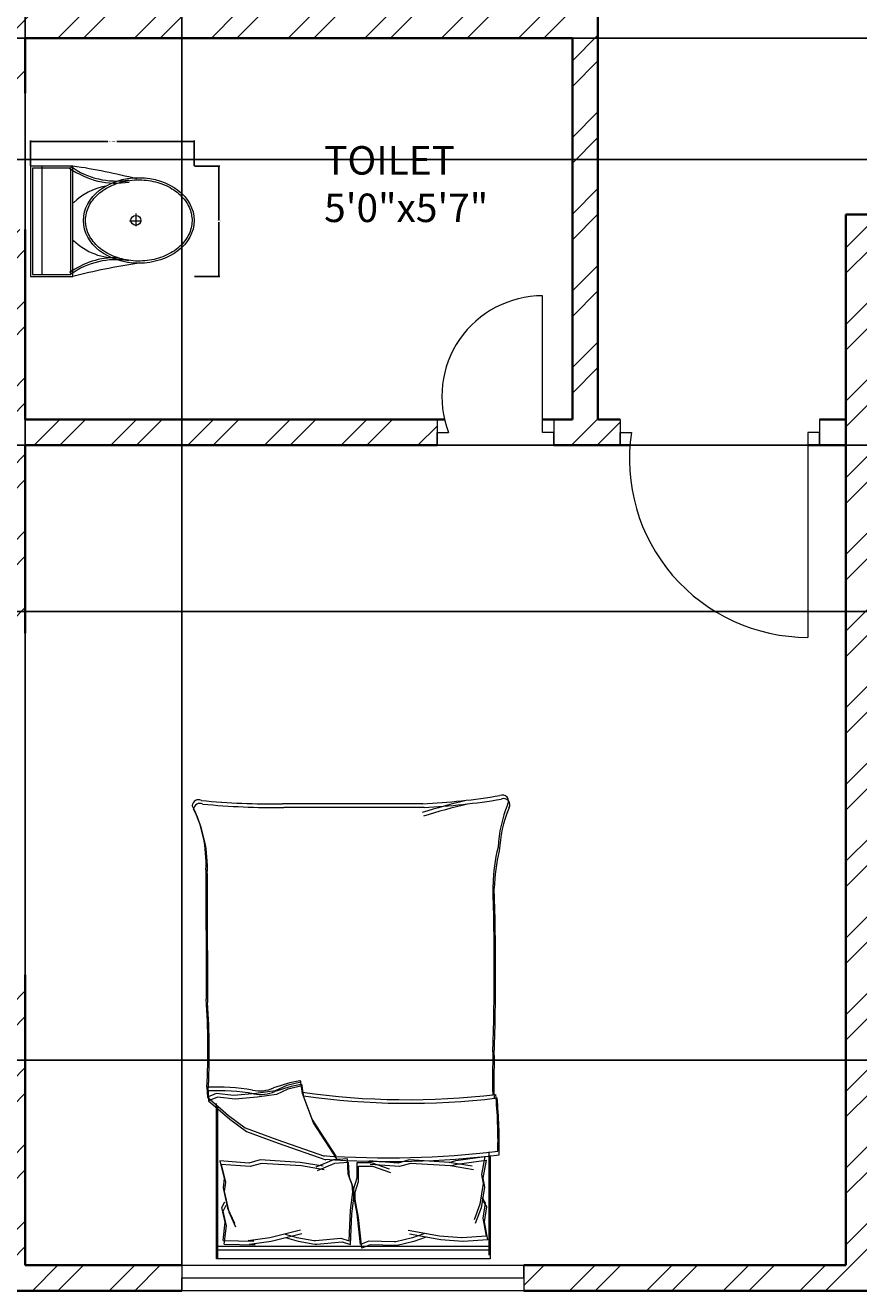
# Model space of a CAD drawing. Units: inches. Extents: x 1965 to 2673, y 1802 to 2669.
# Tile 3 of 16: x 2052 to 2198, y 1932 to 2154. Entities that reach past the tile are written whole.
import ezdxf

# ---------------------------------------------------------------- set-up
doc = ezdxf.new("R2010")
doc.units = ezdxf.units.IN
for name, color, linetype, lineweight in [('A-ANNO-DIMS', 2, 'Continuous', 18), ('A-AREA-IDEN', 7, 'Continuous', 18), ('A-DOOR', 11, 'Continuous', 18), ('A-FLOR-FIXT', 9, 'Continuous', 18), ('A-FURN', 8, 'Continuous', 13), ('A-GLAZ', 181, 'Continuous', 18), ('A-WALL', 7, 'Continuous', 35), ('A-WALL-PATT', 252, 'Continuous', 13)]:
    doc.layers.add(name, color=color, linetype=linetype, lineweight=lineweight)
doc.styles.get("Standard").update_dxf_attribs({"font": 'arial.ttf'})
doc.dimstyles.get("Standard").update_dxf_attribs({"dimtxt": 0.18, "dimasz": 0.18, "dimexe": 0.18, "dimexo": 0.0625, "dimgap": 0.09, "dimtad": 0, "dimtih": 1, "dimtoh": 1, "dimdec": 4, "dimzin": 0, "dimdsep": 46, "dimtxsty": 'Standard', "dimcen": 0.09, "dimadec": 0, "dimazin": 0, "dimtfac": 1, "dimtdec": 4, "dimtofl": 0, "dimtmove": 0, "dimatfit": 3, "dimfxl": 1, "dimtolj": 1, "dimtzin": 0, "dimarcsym": 0})

# ---------------------------------------------------------------- blocks, each defined once
blk = doc.blocks.new('A$C31115884')
for p, q in [((283.1, 497.7), (223.4, 497.7)), ((257.5, 466.4), (257.5, 523.2)), ((0, 200), (0, 0)), ((520, 200), (0, 200)), ((10, 190), (10, 10)), ((510, 190), (10, 190)), ((510, 10), (510, 190)), ((520, 0), (520, 200)), ((510, 54.5), (0, 54.5)), ((10, 10), (510, 10)), ((0, 0), (520, 0))]:
    blk.add_line(p, q)
blk.add_circle((255.6, 496.4), 23.6)
for centre, radius, start, end in [((2777.7, -204.6), 2807, 165.4549, 171.71327), ((3237, 905), 2807, 188.28673, 194.5451), ((-294.5, 403.3), 364.7, 324.20913, 9.34987), ((-294.5, 403.3), 374.7, 324.20913, 9.34987), ((139.5, 406.2), 293.5, 315.84364, 2.65635), ((805.8, 403.3), 364.7, 170.65013, 215.79087), ((805.8, 403.3), 374.7, 179.20365, 215.79087), ((383.6, 406.2), 293.5, 190.27735, 224.15636)]:
    blk.add_arc(centre, radius, start, end)
blk.add_ellipse((256.2, 509.9), major_axis=(0, -260.7), ratio=0.772727)
blk.add_open_spline([(256.2, 259.2), (263.1, 259.2), (270, 259.7), (287.8, 262.3), (298.7, 265.1), (319.9, 273.1), (330.2, 278.4), (350.1, 291.1), (359.7, 298.7), (377.7, 315.9), (386.2, 325.5), (401.7, 346.6), (408.8, 358.1), (421.3, 382.5), (426.8, 395.5), (435.9, 422.4), (439.5, 436.4), (444.8, 465.1), (446.5, 479.7), (447.9, 509.2), (447.6, 524), (445, 553.3), (442.7, 567.8), (436.3, 596), (432.1, 609.7), (421.9, 636), (416, 648.6), (402.5, 672.1), (395, 683), (378.6, 703), (369.8, 712.1), (351.1, 728), (341.3, 734.8), (320.9, 746.2), (310.4, 750.7), (288.9, 757.3), (278, 759.4), (256, 761), (245, 760.6), (223.1, 757.2), (212.3, 754.3), (191.1, 746.1), (180.8, 740.7), (160.9, 727.8), (151.4, 720.1), (133.5, 702.7), (125.1, 693), (109.6, 671.7), (102.6, 660.2), (90.2, 635.7), (84.9, 622.7), (76, 595.6), (72.4, 581.6), (67.2, 552.9), (65.6, 538.2), (64.4, 508.8), (64.8, 494), (67.5, 464.7), (69.9, 450.2), (76.6, 422), (80.8, 408.3), (91.1, 382.2), (97.2, 369.7), (110.8, 346.3), (118.4, 335.4), (134.8, 315.6), (143.7, 306.7), (162.4, 290.9), (172.3, 284.2), (192.8, 273), (203.3, 268.6), (224.8, 262.2), (235.8, 260.2), (249.9, 259.3), (253, 259.2), (256.2, 259.2)], degree=3, knots=[0, 0, 0, 0, 0.110105, 0.110105, 0.285049, 0.285049, 0.459994, 0.459994, 0.634938, 0.634938, 0.809882, 0.809882, 0.984827, 0.984827, 1.159771, 1.159771, 1.334715, 1.334715, 1.50966, 1.50966, 1.684604, 1.684604, 1.859549, 1.859549, 2.034493, 2.034493, 2.209437, 2.209437, 2.384382, 2.384382, 2.559326, 2.559326, 2.73427, 2.73427, 2.909215, 2.909215, 3.084159, 3.084159, 3.259103, 3.259103, 3.434048, 3.434048, 3.608992, 3.608992, 3.783936, 3.783936, 3.958881, 3.958881, 4.133825, 4.133825, 4.30877, 4.30877, 4.483714, 4.483714, 4.658658, 4.658658, 4.833603, 4.833603, 5.008547, 5.008547, 5.183491, 5.183491, 5.358436, 5.358436, 5.53338, 5.53338, 5.708324, 5.708324, 5.883269, 5.883269, 6.058213, 6.058213, 6.233158, 6.233158, 6.283185, 6.283185, 6.283185, 6.283185])
blk = doc.blocks.new('BED-DOUBLE')
for p, q in [((3.47, 63.33), (3.47, 81.44)), ((3.47, 63.33), (3.47, 81.44)), ((3.47, 81.44), (51.49, 81.44)), ((3.7, 62.69), (3.7, 80.8)), ((3.7, 62.69), (3.7, 80.8)), ((51.26, 81.44), (51.26, 54.83)), ((51.26, 81.44), (51.26, 54.83)), ((51.49, 81.44), (51.49, 80.8)), ((51.49, 80.8), (51.49, 54.19)), ((51.49, 80.8), (51.49, 54.19)), ((3.47, 79.91), (51.26, 79.91)), ((3.47, 79.91), (51.26, 79.91)), ((3.7, 79.27), (51.49, 79.27)), ((3.7, 79.27), (51.49, 79.27)), ((3.89, 78.1), (8.17, 78.43)), ((3.89, 78.1), (8.17, 78.43)), ((3.89, 78.12), (4.47, 74.94)), ((3.89, 78.12), (4.47, 74.94)), ((4.12, 77.46), (8.4, 77.79)), ((4.12, 77.46), (8.4, 77.79)), ((8.17, 78.43), (8.28, 78.41)), ((8.17, 78.43), (8.28, 78.41)), ((8.28, 78.41), (12.1, 78.12)), ((8.28, 78.41), (12.1, 78.12)), ((8.4, 77.79), (8.51, 77.77)), ((8.4, 77.79), (8.51, 77.77)), ((12.1, 78.12), (17.6, 77.11)), ((12.1, 78.12), (17.6, 77.11)), ((14.85, 77.69), (16.87, 78.41)), ((14.85, 77.69), (16.87, 78.41)), ((16.87, 78.41), (19.76, 79.14)), ((16.87, 78.41), (19.76, 79.14)), ((17.1, 77.77), (19.99, 78.5)), ((17.1, 77.77), (19.99, 78.5)), ((19.76, 79.14), (20.09, 79.14)), ((19.76, 79.14), (20.09, 79.14)), ((19.99, 78.5), (20.31, 78.5)), ((19.99, 78.5), (20.31, 78.5)), ((20.09, 79.14), (24.53, 78.99)), ((20.09, 79.14), (24.53, 78.99)), ((20.31, 78.5), (24.76, 78.35)), ((20.31, 78.5), (24.76, 78.35)), ((24.53, 78.99), (25.98, 79.57)), ((24.53, 78.99), (25.98, 79.57)), ((24.76, 78.35), (26.21, 78.93)), ((24.76, 78.35), (26.21, 78.93)), ((25.98, 79.57), (26.56, 74.22)), ((25.98, 79.57), (26.56, 74.22)), ((26.21, 78.93), (26.78, 73.58)), ((26.21, 78.93), (26.78, 73.58)), ((27.97, 78.95), (27.73, 73.57)), ((27.97, 78.95), (27.73, 73.57)), ((28.2, 78.31), (27.96, 72.93)), ((28.2, 78.31), (27.96, 72.93)), ((29.45, 78.46), (27.97, 78.95)), ((29.45, 78.46), (27.97, 78.95)), ((29.68, 77.82), (28.2, 78.31)), ((29.68, 77.82), (28.2, 78.31)), ((33.88, 78.88), (29.45, 78.46)), ((33.88, 78.88), (29.45, 78.46)), ((34.11, 78.24), (29.68, 77.82)), ((34.11, 78.24), (29.68, 77.82)), ((34.2, 78.9), (33.88, 78.88)), ((34.2, 78.9), (33.88, 78.88)), ((34.43, 78.26), (34.11, 78.24)), ((34.43, 78.26), (34.11, 78.24)), ((37.13, 78.36), (34.2, 78.9)), ((37.13, 78.36), (34.2, 78.9)), ((37.36, 77.72), (34.43, 78.26)), ((37.36, 77.72), (34.43, 78.26)), ((41.91, 78.37), (36.49, 77.02)), ((41.91, 78.37), (36.49, 77.02)), ((39.2, 77.77), (37.13, 78.36)), ((39.19, 77.77), (37.13, 78.36)), ((45.71, 78.9), (41.91, 78.37)), ((45.71, 78.9), (41.91, 78.37)), ((45.94, 78.26), (42.14, 77.73)), ((45.94, 78.26), (42.14, 77.73)), ((50.11, 78.88), (44.7, 78.98)), ((44.7, 78.98), (45.71, 78.9)), ((50.11, 78.88), (44.7, 78.98)), ((44.7, 78.98), (45.71, 78.9)), ((50.34, 78.24), (44.93, 78.34)), ((44.93, 78.34), (45.94, 78.26)), ((50.34, 78.24), (44.93, 78.34)), ((44.93, 78.34), (45.94, 78.26)), ((50.11, 78.88), (49.73, 75.67)), ((50.11, 78.88), (49.73, 75.67)), ((50.34, 78.24), (49.96, 75.03)), ((50.34, 78.24), (49.96, 75.03)), ((4.12, 77.49), (4.7, 74.3)), ((4.12, 77.49), (4.7, 74.3)), ((8.51, 77.77), (12.33, 77.49)), ((8.51, 77.77), (12.33, 77.49)), ((12.33, 77.49), (17.82, 76.47)), ((12.33, 77.49), (17.82, 76.47)), ((15.08, 77.05), (17.1, 77.77)), ((15.08, 77.05), (17.1, 77.77)), ((42.14, 77.73), (36.72, 76.38)), ((42.14, 77.73), (36.72, 76.38)), ((39.42, 77.13), (37.36, 77.72)), ((39.42, 77.13), (37.36, 77.72)), ((49.3, 73.18), (48.12, 75.86)), ((49.3, 73.18), (48.12, 75.86)), ((49.73, 75.67), (50.32, 73.1)), ((49.73, 75.67), (50.32, 73.1)), ((4.47, 74.94), (4.03, 72.34)), ((4.47, 74.94), (4.03, 72.34)), ((4.7, 74.3), (4.26, 71.7)), ((4.7, 74.3), (4.26, 71.7)), ((5.05, 72.49), (6.06, 75.23)), ((5.05, 72.49), (6.06, 75.23)), ((5.27, 71.85), (6.29, 74.59)), ((5.27, 71.85), (6.29, 74.59)), ((26.56, 74.22), (27.13, 71.04)), ((26.56, 74.22), (27.13, 71.04)), ((26.78, 73.58), (27.36, 70.4)), ((26.78, 73.58), (27.36, 70.4)), ((27.73, 73.57), (27.35, 70.36)), ((27.73, 73.57), (27.35, 70.36)), ((49.53, 72.54), (48.35, 75.22)), ((49.53, 72.54), (48.35, 75.22)), ((49.96, 75.03), (50.55, 72.46)), ((49.96, 75.03), (50.55, 72.46)), ((4.03, 72.34), (4.61, 71.33)), ((4.03, 72.34), (4.61, 71.33)), ((4.26, 71.7), (4.84, 70.69)), ((4.26, 71.7), (4.84, 70.69)), ((4.47, 68.87), (5.05, 72.49)), ((4.47, 68.87), (5.05, 72.49)), ((4.7, 68.23), (5.27, 71.85)), ((4.7, 68.23), (5.27, 71.85)), ((27.96, 72.93), (27.58, 69.72)), ((27.96, 72.93), (27.58, 69.72)), ((50.11, 69.61), (49.3, 73.18)), ((50.11, 69.61), (49.3, 73.18)), ((50.34, 68.97), (49.53, 72.54)), ((50.34, 68.97), (49.53, 72.54)), ((50.32, 73.1), (49.81, 72.06)), ((50.32, 73.1), (49.81, 72.06)), ((50.55, 72.46), (50.04, 71.42)), ((50.55, 72.46), (50.04, 71.42)), ((27.13, 69.74), (26.56, 67.86)), ((27.13, 69.74), (26.56, 67.86)), ((27.36, 69.1), (26.78, 67.22)), ((27.36, 69.1), (26.78, 67.22)), ((27.13, 71.04), (27.13, 69.74)), ((27.13, 71.04), (27.13, 69.74)), ((27.35, 70.36), (27.43, 69.06)), ((27.35, 70.36), (27.43, 69.06)), ((27.36, 70.4), (27.36, 69.1)), ((27.36, 70.4), (27.36, 69.1)), ((27.43, 69.06), (28.13, 67.22)), ((27.43, 69.06), (28.13, 67.22)), ((27.58, 69.72), (27.66, 68.42)), ((27.58, 69.72), (27.66, 68.42)), ((49.92, 68.01), (50.11, 69.61)), ((49.92, 68.01), (50.11, 69.61)), ((50.15, 67.37), (50.34, 68.97)), ((50.15, 67.37), (50.34, 68.97)), ((4.18, 64.1), (4.76, 67.28)), ((4.18, 64.1), (4.76, 67.28)), ((4.76, 67.28), (4.47, 68.87)), ((4.76, 67.28), (4.47, 68.87)), ((4.99, 66.64), (4.7, 68.23)), ((4.99, 66.64), (4.7, 68.23)), ((26.56, 67.86), (26.56, 65.18)), ((26.56, 67.86), (26.56, 65.18)), ((26.78, 67.22), (26.78, 64.54)), ((26.78, 67.22), (26.78, 64.54)), ((27.66, 68.42), (28.35, 66.58)), ((27.66, 68.42), (28.35, 66.58)), ((28.13, 67.22), (28.29, 64.55)), ((28.13, 67.22), (28.29, 64.55)), ((50.69, 64.87), (49.92, 68.01)), ((50.69, 64.87), (49.92, 68.01)), ((50.92, 64.23), (50.15, 67.37)), ((50.92, 64.23), (50.15, 67.37)), ((9.28, 64.82), (4.18, 64.1)), ((9.28, 64.82), (4.18, 64.1)), ((4.41, 63.46), (4.99, 66.64)), ((4.41, 63.46), (4.99, 66.64)), ((6.38, 65.81), (10.41, 65.15)), ((6.38, 65.81), (10.41, 65.15)), ((6.6, 65.17), (10.64, 64.51)), ((6.61, 65.17), (10.64, 64.51)), ((10.41, 65.15), (9.28, 64.82)), ((10.41, 65.15), (9.28, 64.82)), ((10.64, 64.51), (9.5, 64.18)), ((10.64, 64.51), (9.5, 64.18)), ((10.41, 65.15), (17.42, 64.71)), ((10.41, 65.15), (17.42, 64.71)), ((10.64, 64.51), (17.65, 64.08)), ((10.64, 64.51), (17.65, 64.08)), ((17.42, 64.71), (19.38, 65.27)), ((17.42, 64.71), (19.38, 65.27)), ((17.65, 64.08), (19.61, 64.63)), ((17.65, 64.08), (19.61, 64.63)), ((19.38, 65.27), (24.51, 64.87)), ((19.38, 65.27), (24.51, 64.87)), ((19.61, 64.63), (24.74, 64.23)), ((19.61, 64.63), (24.74, 64.23)), ((24.1, 65.18), (20.95, 66.27)), ((24.1, 65.18), (20.95, 66.27)), ((24.33, 64.54), (21.18, 65.63)), ((24.33, 64.54), (21.18, 65.63)), ((26.56, 65.18), (24.1, 65.18)), ((26.56, 65.18), (24.1, 65.18)), ((26.78, 64.54), (24.33, 64.54)), ((26.78, 64.54), (24.33, 64.54)), ((28.29, 64.55), (30.75, 64.7)), ((28.29, 64.55), (30.75, 64.7)), ((28.35, 66.58), (28.52, 63.91)), ((28.35, 66.58), (28.52, 63.91)), ((30.75, 64.7), (33.82, 65.99)), ((30.75, 64.7), (33.82, 65.99)), ((30.97, 64.06), (34.04, 65.35)), ((30.97, 64.06), (34.04, 65.35)), ((32.56, 65.81), (36.59, 65.15)), ((32.56, 65.81), (36.59, 65.15)), ((32.79, 65.17), (36.82, 64.51)), ((32.79, 65.17), (36.82, 64.51)), ((36.59, 65.15), (43.6, 64.71)), ((36.59, 65.15), (43.6, 64.71)), ((36.82, 64.51), (43.83, 64.08)), ((36.82, 64.51), (43.83, 64.08)), ((43.6, 64.71), (45.56, 65.27)), ((43.6, 64.71), (45.56, 65.27)), ((43.83, 64.08), (45.79, 64.63)), ((43.83, 64.08), (45.79, 64.63)), ((45.56, 65.27), (50.69, 64.87)), ((45.56, 65.27), (50.69, 64.87)), ((45.79, 64.63), (50.92, 64.23)), ((45.79, 64.63), (50.92, 64.23)), ((9.5, 64.18), (4.41, 63.46)), ((9.5, 64.18), (4.41, 63.46)), ((28.52, 63.91), (30.97, 64.06)), ((28.52, 63.91), (30.97, 64.06)), ((30.25, 64.06), (34.44, 57.56)), ((30.25, 64.06), (34.44, 57.56)), ((30.48, 63.42), (34.67, 56.92)), ((30.48, 63.42), (34.67, 56.92)), ((40.64, 61.12), (32.3, 64.06)), ((40.64, 61.12), (32.3, 64.06)), ((40.87, 60.48), (32.53, 63.42)), ((40.87, 60.48), (32.53, 63.42)), ((46.21, 59.11), (40.64, 61.12)), ((46.21, 59.11), (40.64, 61.12)), ((46.44, 58.47), (40.87, 60.48)), ((46.44, 58.47), (40.87, 60.48)), ((49.16, 56.95), (46.21, 59.11)), ((49.16, 56.95), (46.21, 59.11)), ((49.39, 56.31), (46.44, 58.47)), ((49.39, 56.31), (46.44, 58.47)), ((34.44, 57.56), (36.15, 53.08)), ((34.44, 57.56), (36.15, 53.08)), ((34.67, 56.92), (36.38, 52.44)), ((34.67, 56.92), (36.38, 52.44)), ((52.86, 53.69), (49.16, 56.95)), ((52.86, 53.69), (49.16, 56.95)), ((53.09, 53.06), (49.39, 56.31)), ((53.09, 53.06), (49.39, 56.31)), ((44.36, 53.08), (48.23, 53.39)), ((44.36, 53.08), (48.23, 53.39)), ((48.23, 53.39), (51.33, 53.08)), ((48.23, 53.39), (51.33, 53.08)), ((51.33, 53.08), (52.86, 53.69)), ((51.33, 53.08), (52.86, 53.69)), ((52.94, 51.95), (52.86, 53.69, 3.87)), ((52.94, 51.95), (52.86, 53.69, 3.87)), ((36.15, 53.08), (36.46, 51.06)), ((36.15, 53.08), (36.46, 51.06)), ((36.38, 52.44), (36.69, 50.42)), ((36.38, 52.44), (36.69, 50.42)), ((36.46, 51.06), (38.94, 51.68)), ((36.46, 51.06), (38.94, 51.68)), ((38.94, 51.68), (40.95, 52.61)), ((38.94, 51.68), (40.95, 52.61)), ((39.16, 51.04), (41.18, 51.97)), ((39.16, 51.04), (41.18, 51.97)), ((40.95, 52.61), (44.36, 53.08)), ((40.95, 52.61), (44.36, 53.08)), ((41.18, 51.97), (44.58, 52.44)), ((41.18, 51.97), (44.58, 52.44)), ((44.58, 52.44), (48.46, 52.75)), ((44.58, 52.44), (48.46, 52.75)), ((48.46, 52.75), (51.55, 52.44)), ((48.46, 52.75), (51.55, 52.44)), ((51.55, 52.44), (53.09, 53.06)), ((51.55, 52.44), (53.09, 53.06)), ((53.17, 51.31), (53.09, 53.06, 3.87)), ((53.17, 51.31), (53.09, 53.06, 3.87)), ((36.69, 50.42), (39.16, 51.04)), ((36.69, 50.42), (39.16, 51.04)), ((15.06, 2.2), (39.67, 2.2)), ((15.06, 2.2), (39.67, 2.2)), ((15.29, 1.56), (39.9, 1.56)), ((15.29, 1.56), (39.9, 1.56))]:
    blk.add_line(p, q)
for centre, radius, start, end in [((85.16, 61.34), 83.31, 178.7218, 185.604), ((85.16, 61.34), 83.31, 178.7218, 185.604), ((21.35, -100.61), 164.97, 86.0865, 96.7821), ((21.35, -100.61), 164.97, 86.0865, 96.7821), ((85.39, 60.71), 83.31, 178.7218, 185.604), ((85.38, 60.71), 83.31, 178.7218, 185.604), ((21.58, -101.25), 164.97, 86.0865, 96.7821), ((21.58, -101.25), 164.97, 86.0865, 96.7821), ((17.75, -74.88), 129.02, 81.7845, 96.9006), ((17.75, -74.88), 129.02, 81.7845, 96.9006), ((17.98, -75.51), 129.02, 81.7845, 96.9006), ((17.98, -75.51), 129.02, 81.7845, 96.9006), ((-167.31, 50.27), 170.11, 358.4762, 1.0082), ((-167.31, 50.27), 170.11, 358.4762, 1.0082), ((-167.08, 49.63), 170.11, 358.4762, 1.0082), ((-167.08, 49.63), 170.11, 358.4762, 1.0082), ((31.15, 79.96), 29.65, 280.6617, 289.8806), ((31.15, 79.96), 29.65, 280.6617, 289.8806), ((31.38, 79.32), 29.65, 280.6617, 289.8806), ((31.38, 79.32), 29.65, 280.6617, 289.8806), ((43.74, 46.37), 6.22, 78.6608, 113.7384), ((43.74, 46.37), 6.22, 78.6608, 113.7384), ((43.97, 45.74), 6.22, 78.6608, 113.7384), ((43.97, 45.74), 6.22, 78.6608, 113.7384), ((51.32, 88.1), 36.18, 259.8763, 272.5657), ((51.32, 88.1), 36.18, 259.8763, 272.5657), ((51.55, 87.46), 36.18, 259.8763, 272.5657), ((51.55, 87.46), 36.18, 259.8763, 272.5657), ((182.26, 45.13), 129.5, 176.9791, 183.8365), ((182.26, 45.13), 129.5, 176.9791, 183.8365), ((182.49, 44.49), 129.5, 176.9791, 183.8365), ((182.49, 44.49), 129.5, 176.9791, 183.8365), ((36.63, 51), 0.185, 160.2464, 271.1377), ((36.63, 51), 0.185, 160.2464, 271.1377), ((36.86, 50.36), 0.185, 160.2464, 271.1377), ((36.86, 50.36), 0.185, 160.2464, 271.1377), ((484.82, 30.83), 482.31, 178.2277, 181.7185), ((484.82, 30.83), 482.31, 178.2277, 181.7185), ((485.05, 30.19), 482.31, 178.2277, 181.7185), ((485.05, 30.19), 482.31, 178.2277, 181.7185), ((-4508.75, 13.62), 4561.86, 0.00217, 0.28689), ((-4508.75, 13.62), 4561.86, 0.00217, 0.28689), ((-4508.52, 12.98), 4561.86, 0.00217, 0.28689), ((-4508.52, 12.98), 4561.86, 0.00217, 0.28689), ((-26.9, 16.93), 29.63, 346.0648, 358.9113), ((-26.9, 16.93), 29.63, 346.0648, 358.9113), ((-26.68, 16.29), 29.63, 346.0648, 358.9113), ((-26.68, 16.29), 29.63, 346.0648, 358.9113), ((76.15, 12.77), 23.07, 177.4714, 206.4681), ((76.15, 12.77), 23.07, 177.4714, 206.4681), ((76.38, 12.14), 23.07, 177.4714, 206.4681), ((76.38, 12.14), 23.07, 177.4714, 206.4681), ((-21.66, 11.17), 23.56, 337.9751, 356.652), ((-21.66, 11.17), 23.56, 337.9751, 356.652), ((-21.44, 10.53), 23.56, 337.9751, 356.652), ((-21.44, 10.53), 23.56, 337.9751, 356.652), ((1.08, 1.72), 1.09, 146.1736, 293.4781), ((1.08, 1.72), 1.09, 146.1736, 293.4781), ((-17.23, 105.15), 106.46, 283.3832, 287.7053), ((-17.23, 105.15), 106.46, 283.3832, 287.7053), ((-17, 104.51), 106.46, 283.3832, 287.7053), ((-17, 104.51), 106.46, 283.3832, 287.7053), ((54.4, 2.57), 1.1, 242.6588, 356.02), ((54.4, 2.57), 1.1, 242.6588, 356.02), ((1.31, 1.08), 1.09, 146.1736, 293.4781), ((1.31, 1.08), 1.09, 146.1736, 293.4781), ((21.42, -119.4), 121.76, 92.9958, 99.4091), ((21.42, -119.4), 121.76, 92.9958, 99.4091), ((21.65, -120.04), 121.76, 92.9958, 99.4091), ((21.65, -120.04), 121.76, 92.9958, 99.4091), ((41.15, -130.84), 133.04, 84.4998, 90.6351), ((41.15, -130.84), 133.04, 84.4998, 90.6351), ((41.38, -131.48), 133.04, 84.4998, 90.6351), ((41.37, -131.48), 133.04, 84.4998, 90.6351), ((54.63, 1.93), 1.1, 242.6588, 356.02), ((54.63, 1.93), 1.1, 242.6588, 356.02)]:
    blk.add_arc(centre, radius, start, end)
blk = doc.blocks.new('WIN-60IN')
for p, q in [((0, 4.5), (0, 0)), ((0, 4.5), (60, 4.5)), ((60, 2.25), (60, 4.5)), ((60, 4.5), (60, 0)), ((0, 0), (0, 2.25)), ((0, 2.25), (60, 2.25)), ((60, 0), (0, 0))]:
    blk.add_line(p, q)
blk = doc.blocks.new('*D17')
at = {"layer": 'A-ANNO-DIMS', "color": 0, "lineweight": -2, "transparency": 16777216}
for p, q in [((2052.5, 2129.17), (2052.5, 2133.6)), ((2052.68, 2133.42), (2066.08, 2133.42)), ((2081.04, 2133.42), (2067.64, 2133.42)), ((2081.22, 2129.17), (2081.22, 2133.6))]:
    blk.add_line(p, q, dxfattribs=at)
at = {"layer": 'A-ANNO-DIMS', "color": 0, "transparency": 16777216}
for points in [[(2052.68, 2133.45), (2052.68, 2133.39), (2052.5, 2133.42)], [(2081.04, 2133.45), (2081.04, 2133.39), (2081.22, 2133.42)]]:
    blk.add_solid(points, dxfattribs=at)
at = {"layer": 'Defpoints', "color": 0, "transparency": 16777216}
for p in [(2081.22, 2133.42), (2052.5, 2129.11), (2081.22, 2129.11)]:
    blk.add_point(p, dxfattribs=at)
at = {"layer": 'A-ANNO-DIMS', "color": 0, "transparency": 16777216, "insert": (2066.86, 2133.42), "char_height": 0.18, "attachment_point": 5}
blk.add_mtext('\\A1;WC 29 TYP.', dxfattribs=at)
blk = doc.blocks.new('*D18')
at = {"layer": 'A-ANNO-DIMS', "color": 0, "lineweight": -2, "transparency": 16777216}
for p, q in [((2081.28, 2129.11), (2085.71, 2129.11)), ((2085.53, 2128.93), (2085.53, 2119.6)), ((2085.53, 2109.91), (2085.53, 2119.24)), ((2081.28, 2109.73), (2085.71, 2109.73))]:
    blk.add_line(p, q, dxfattribs=at)
at = {"layer": 'A-ANNO-DIMS', "color": 0, "transparency": 16777216}
for points in [[(2085.5, 2128.93), (2085.56, 2128.93), (2085.53, 2129.11)], [(2085.5, 2109.91), (2085.56, 2109.91), (2085.53, 2109.73)]]:
    blk.add_solid(points, dxfattribs=at)
at = {"layer": 'Defpoints', "color": 0, "transparency": 16777216}
for p in [(2081.22, 2129.11), (2081.22, 2109.73), (2085.53, 2109.73)]:
    blk.add_point(p, dxfattribs=at)
at = {"layer": 'A-ANNO-DIMS', "color": 0, "transparency": 16777216, "insert": (2085.53, 2119.42), "char_height": 0.18, "attachment_point": 5}
blk.add_mtext('\\A1;19 TYP.', dxfattribs=at)
blk = doc.blocks.new('*D39')
at = {"layer": 'A-ANNO-DIMS', "color": 0, "lineweight": -2, "transparency": 16777216}
for p, q in [((2051.59, 1936.15), (2051.59, 2600.5)), ((2079.05, 1936.15), (2079.05, 2600.5)), ((2051.77, 2600.32), (2064.93, 2600.32)), ((2078.87, 2600.32), (2065.72, 2600.32))]:
    blk.add_line(p, q, dxfattribs=at)
at = {"layer": 'A-ANNO-DIMS', "color": 0, "transparency": 16777216}
for points in [[(2051.77, 2600.35), (2051.77, 2600.29), (2051.59, 2600.32)], [(2078.87, 2600.35), (2078.87, 2600.29), (2079.05, 2600.32)]]:
    blk.add_solid(points, dxfattribs=at)
at = {"layer": 'Defpoints', "color": 0, "transparency": 16777216}
for p in [(2079.05, 2600.32), (2051.59, 1936.09), (2079.05, 1936.09)]:
    blk.add_point(p, dxfattribs=at)
at = {"layer": 'A-ANNO-DIMS', "color": 0, "transparency": 16777216, "insert": (2065.32, 2600.32), "char_height": 0.18, "attachment_point": 5}
blk.add_mtext('\\A1;27.46', dxfattribs=at)
blk = doc.blocks.new('*D45')
at = {"layer": 'A-ANNO-DIMS', "color": 0, "lineweight": -2, "transparency": 16777216}
for p, q in [((2573.53, 2080.09), (2012.19, 2080.09)), ((2012.37, 2079.91), (2012.37, 2065.68)), ((2012.37, 2051.08), (2012.37, 2065.31)), ((2573.53, 2050.9), (2012.19, 2050.9))]:
    blk.add_line(p, q, dxfattribs=at)
at = {"layer": 'A-ANNO-DIMS', "color": 0, "transparency": 16777216}
for points in [[(2012.34, 2079.91), (2012.4, 2079.91), (2012.37, 2080.09)], [(2012.34, 2051.08), (2012.4, 2051.08), (2012.37, 2050.9)]]:
    blk.add_solid(points, dxfattribs=at)
at = {"layer": 'Defpoints', "color": 0, "transparency": 16777216}
for p in [(2012.37, 2080.09), (2573.59, 2080.09), (2573.59, 2050.9)]:
    blk.add_point(p, dxfattribs=at)
at = {"layer": 'A-ANNO-DIMS', "color": 0, "transparency": 16777216, "insert": (2012.37, 2065.49), "char_height": 0.18, "attachment_point": 5}
blk.add_mtext('\\A1;29.19', dxfattribs=at)
blk = doc.blocks.new('*D46')
at = {"layer": 'A-ANNO-DIMS', "color": 0, "lineweight": -2, "transparency": 16777216}
for p, q in [((2573.53, 2151.59), (2012.19, 2151.59)), ((2012.37, 2151.41), (2012.37, 2141.12)), ((2012.37, 2130.47), (2012.37, 2140.76)), ((2573.53, 2130.29), (2012.19, 2130.29))]:
    blk.add_line(p, q, dxfattribs=at)
at = {"layer": 'A-ANNO-DIMS', "color": 0, "transparency": 16777216}
for points in [[(2012.34, 2151.41), (2012.4, 2151.41), (2012.37, 2151.59)], [(2012.34, 2130.47), (2012.4, 2130.47), (2012.37, 2130.29)]]:
    blk.add_solid(points, dxfattribs=at)
at = {"layer": 'Defpoints', "color": 0, "transparency": 16777216}
for p in [(2012.37, 2151.59), (2573.59, 2151.59), (2573.59, 2130.29)]:
    blk.add_point(p, dxfattribs=at)
at = {"layer": 'A-ANNO-DIMS', "color": 0, "transparency": 16777216, "insert": (2012.37, 2140.94), "char_height": 0.18, "attachment_point": 5}
blk.add_mtext('\\A1;21.3', dxfattribs=at)
blk = doc.blocks.new('*D51')
at = {"layer": 'A-ANNO-DIMS', "color": 0, "lineweight": -2, "transparency": 16777216}
for p, q in [((2388.03, 2080.09), (2012.19, 2080.09)), ((2012.37, 2079.91), (2012.37, 2026.27)), ((2012.37, 1972.27), (2012.37, 2025.91)), ((2388.03, 1972.09), (2012.19, 1972.09))]:
    blk.add_line(p, q, dxfattribs=at)
at = {"layer": 'A-ANNO-DIMS', "color": 0, "transparency": 16777216}
for points in [[(2012.34, 2079.91), (2012.4, 2079.91), (2012.37, 2080.09)], [(2012.34, 1972.27), (2012.4, 1972.27), (2012.37, 1972.09)]]:
    blk.add_solid(points, dxfattribs=at)
at = {"layer": 'Defpoints', "color": 0, "transparency": 16777216}
for p in [(2012.37, 2080.09), (2388.09, 2080.09), (2388.09, 1972.09)]:
    blk.add_point(p, dxfattribs=at)
at = {"layer": 'A-ANNO-DIMS', "color": 0, "transparency": 16777216, "insert": (2012.37, 2026.09), "char_height": 0.18, "attachment_point": 5}
blk.add_mtext('\\A1;108', dxfattribs=at)

msp = doc.modelspace()

# ---------------------------------------------------------------- hatches: boundary and pattern name
at = {"layer": 'A-WALL-PATT'}
h = msp.add_hatch(dxfattribs=at)
h.set_pattern_fill('ANSI32', color=256)
h.paths.add_polyline_path([(2051.5927, 2561.0914), (2076.7559, 2561.0914), (2076.7559, 2563.3414), (2076.7559, 2565.5914), (2047.0927, 2565.5914), (2047.0927, 2518.3824), (2051.5927, 2518.3824)])
h.paths.add_polyline_path([(2051.5927, 2458.3824), (2049.3427, 2458.3824), (2047.0927, 2458.3824), (2047.0927, 2412.5914), (2248.0927, 2412.5914), (2248.0927, 2268.5914), (2252.5927, 2268.5914), (2252.5927, 2412.5914), (2252.5927, 2421.0404), (2250.3427, 2421.0404), (2248.0927, 2421.0404), (2248.0927, 2417.0914), (2051.5927, 2417.0914)])
h.paths.add_polyline_path([(2211.4933, 2268.5914), (2104.0927, 2268.5914), (2104.0927, 2272.4654), (2101.8427, 2272.4654), (2099.5927, 2272.4654), (2099.5927, 2268.5914), (2051.5927, 2268.5914), (2051.5927, 2264.0914), (2147.5927, 2264.0914), (2147.5927, 2259.8893), (2152.0927, 2259.8893), (2152.0927, 2264.0914), (2211.4933, 2264.0914), (2211.4933, 2266.3414)])
h.paths.add_polyline_path([(2104.0927, 2376.0914), (2099.5927, 2376.0914), (2047.0927, 2376.0914), (2047.0927, 2333.0682), (2051.5927, 2333.0682), (2051.5927, 2371.5914), (2099.5927, 2371.5914), (2099.5927, 2293.6123), (2104.0927, 2293.6123)], flags=17)
h.paths.add_polyline_path([(2051.5927, 2309.0682), (2047.0927, 2309.0682), (2047.0927, 2233.5821), (2051.5927, 2233.5821)])
h.paths.add_polyline_path([(2104.0927, 2412.5914), (2099.5927, 2412.5914), (2099.5927, 2376.0914), (2104.0927, 2376.0914)], flags=17)
h.paths.add_polyline_path([(2290.1254, 2268.5914), (2242.4924, 2268.5914), (2242.4924, 2264.0914), (2290.1254, 2264.0914), (2290.1254, 2266.3414)])
h.paths.add_polyline_path([(2284.653, 2264.0914), (2280.153, 2264.0914), (2280.153, 2161.6826), (2284.653, 2161.6826)])
h.paths.add_polyline_path([(2578.0927, 2329.4656), (2573.5927, 2329.4656), (2573.5927, 2268.5914), (2525.5927, 2268.5914), (2525.5927, 2271.9222), (2523.3427, 2271.9222), (2521.0927, 2271.9222), (2521.0927, 2268.5914), (2324.2835, 2268.5914), (2324.2835, 2264.0914), (2329.0927, 2264.0914), (2329.0927, 2259.4977), (2333.5927, 2259.4977), (2333.5927, 2264.0914), (2473.0927, 2264.0914), (2473.0927, 2259.9371), (2477.5927, 2259.9371), (2477.5927, 2264.0914), (2573.5927, 2264.0914), (2573.5927, 2235.5751), (2578.0927, 2235.5751)])
h.paths.add_polyline_path([(2377.0927, 2412.5914), (2578.0927, 2412.5914), (2578.0927, 2444.2286), (2575.8427, 2444.2286), (2573.5927, 2444.2286), (2573.5927, 2417.0914), (2429.5927, 2417.0914), (2377.0927, 2417.0914), (2377.0927, 2421.7443), (2372.5927, 2421.7443), (2372.5927, 2268.5914), (2377.0927, 2268.5914)])
h.paths.add_polyline_path([(2525.5927, 2371.5914), (2573.5927, 2371.5914), (2573.5927, 2353.4656), (2578.0927, 2353.4656), (2578.0927, 2376.0914), (2525.5927, 2376.0914), (2521.0927, 2376.0914), (2521.0927, 2290.6472), (2525.5927, 2290.6472)], flags=17)
h.paths.add_polyline_path([(2477.5927, 2236.4106), (2475.3427, 2236.4106), (2473.0927, 2236.4106), (2473.0927, 2084.5914), (2465.3309, 2084.5914), (2465.3309, 2080.0914), (2481.6764, 2080.0914), (2481.6764, 2082.3414), (2481.6764, 2084.5914), (2477.5927, 2084.5914), (2477.5927, 2151.5914), (2573.5927, 2151.5914), (2573.5927, 2130.2907), (2578.0927, 2130.2907), (2578.0927, 2199.5751), (2575.8427, 2199.5751), (2573.5927, 2199.5751), (2573.5927, 2156.0914), (2477.5927, 2156.0914)])
h.paths.add_polyline_path([(2573.5927, 2084.5914), (2505.5513, 2084.5914), (2505.5513, 2080.0914), (2573.5927, 2080.0914)], flags=17)
h.paths.add_polyline_path([(2578.0927, 2106.2907), (2575.8427, 2106.2907), (2573.5927, 2106.2907), (2573.5927, 2050.8986), (2578.0927, 2050.8986)])
h.paths.add_polyline_path([(2578.0927, 1990.8986), (2575.8427, 1990.8986), (2573.5927, 1990.8986), (2573.5927, 1936.0914), (2522.132, 1936.0914), (2522.132, 1931.5914), (2578.0927, 1931.5914)])
h.paths.add_polyline_path([(2462.132, 1936.0914), (2429.5927, 1936.0914), (2429.5927, 2080.0914), (2432.623, 2080.0914), (2432.623, 2082.3414), (2432.623, 2084.5914), (2429.5927, 2084.5914), (2429.5927, 2120.5914), (2333.5927, 2120.5914), (2333.5927, 2229.3125), (2331.3427, 2229.3125), (2329.0927, 2229.3125), (2329.0927, 2116.0914), (2425.0927, 2116.0914), (2425.0927, 1936.0914), (2346.4058, 1936.0914), (2346.4058, 1931.5914), (2462.132, 1931.5914), (2462.132, 1933.8414)])
h.paths.add_polyline_path([(2211.767, 1933.8414), (2211.767, 1936.0914), (2200.0927, 1936.0914), (2200.0927, 2080.0914), (2200.0927, 2116.0914), (2284.653, 2116.0914), (2284.653, 2130.591), (2282.403, 2130.591), (2280.153, 2130.591), (2280.153, 2120.5914), (2200.0927, 2120.5914), (2195.5927, 2120.5914), (2195.5927, 2080.0914), (2195.5927, 1936.0914), (2139.0533, 1936.0914), (2139.0533, 1931.5914), (2211.767, 1931.5914)])
h.paths.add_polyline_path([(2282.2502, 1933.8414), (2282.2502, 1936.0914), (2259.767, 1936.0914), (2259.767, 1931.5914), (2282.2502, 1931.5914)], flags=17)
h.paths.add_polyline_path([(2051.5927, 1987.096), (2049.3427, 1987.096), (2047.0927, 1987.096), (2047.0927, 1931.5914), (2079.0533, 1931.5914), (2079.0533, 1933.8414), (2079.0533, 1936.0914), (2051.5927, 1936.0914)])
h.paths.add_polyline_path([(2051.5927, 2197.5821), (2049.3427, 2197.5821), (2047.0927, 2197.5821), (2047.0927, 2141.952), (2051.5927, 2141.952), (2051.5927, 2151.5914), (2147.5927, 2151.5914), (2147.5927, 2084.5914), (2144.3652, 2084.5914), (2144.3652, 2080.0914), (2155.9662, 2080.0914), (2155.9662, 2082.3414), (2155.9662, 2084.5914), (2152.0927, 2084.5914), (2152.0927, 2239.4921), (2149.8427, 2239.4921), (2147.5927, 2239.4921), (2147.5927, 2156.0914), (2051.5927, 2156.0914)])
h.paths.add_polyline_path([(2051.5927, 2080.0914), (2123.8575, 2080.0914), (2123.8575, 2082.3414), (2123.8575, 2084.5914), (2051.5927, 2084.5914), (2051.5927, 2117.952), (2047.0927, 2117.952), (2047.0927, 2047.096), (2051.5927, 2047.096)])
h = msp.add_hatch(dxfattribs=at)
h.set_pattern_fill('ANSI32', color=256)
h.paths.add_polyline_path([(2210.2316, 2563.3414), (2210.2316, 2565.5914), (2136.7559, 2565.5914), (2136.7559, 2561.0914), (2195.5927, 2561.0914), (2195.5927, 2485.8604), (2200.0927, 2485.8604), (2200.0927, 2561.0914), (2210.2316, 2561.0914)])
h.paths.add_polyline_path([(2285.9734, 2565.5914), (2234.2316, 2565.5914), (2234.2316, 2561.0914), (2248.0927, 2561.0914), (2248.0927, 2462.0914), (2200.0927, 2462.0914), (2200.0927, 2465.2357), (2197.8427, 2465.2357), (2195.5927, 2465.2357), (2195.5927, 2457.5914), (2248.0927, 2457.5914), (2248.0927, 2452.628), (2252.5927, 2452.628), (2252.5927, 2457.5914), (2257.5156, 2457.5914), (2257.5156, 2459.8414), (2257.5156, 2462.0914), (2252.5927, 2462.0914), (2252.5927, 2561.0914), (2285.9734, 2561.0914)])
h.paths.add_polyline_path([(2213.1374, 1872.8885), (2461.061, 1872.8885), (2461.061, 1909.9813), (2213.1374, 1909.9813)], flags=9)
h.paths.add_polyline_path([(2328.4056, 1942.3944), (2340.6089, 1942.3944), (2340.6089, 1952.6979), (2328.4056, 1952.6979)], flags=9)
h.paths.add_polyline_path([(2353.5759, 2030.9808), (2376.6455, 2030.9808), (2376.6455, 2041.2844), (2353.5759, 2041.2844)], flags=9)
h.paths.add_polyline_path([(2289.989, 2074.1041), (2326.916, 2074.1041), (2326.916, 2092.7615), (2289.989, 2092.7615)], flags=9)
h.paths.add_polyline_path([(2497.9, 2052.8638), (2548.3741, 2052.8638), (2548.3741, 2071.5212), (2497.9, 2071.5212)], flags=9)
h.paths.add_polyline_path([(2486.59, 2116.4883), (2515.7475, 2116.4883), (2515.7475, 2135.1456), (2486.59, 2135.1456)], flags=9)
h.paths.add_polyline_path([(2497.3007, 2181.2877), (2530.459, 2181.2877), (2530.459, 2199.945), (2497.3007, 2199.945)], flags=9)
h.paths.add_polyline_path([(2288.237, 2190.3228), (2324.1238, 2190.3228), (2324.1238, 2208.9802), (2288.237, 2208.9802)], flags=9)
h.paths.add_polyline_path([(2350.806, 2127.8307), (2387.733, 2127.8307), (2387.733, 2146.488), (2350.806, 2146.488)], flags=9)
h.paths.add_polyline_path([(2530.3237, 2315.2679), (2559.5563, 2315.2679), (2559.5563, 2333.9252), (2530.3237, 2333.9252)], flags=9)
h.paths.add_polyline_path([(2418.419, 2383.4707), (2468.2894, 2383.4707), (2468.2894, 2402.1281), (2418.419, 2402.1281)], flags=9)
h.paths.add_polyline_path([(2327.4503, 2399.0281), (2364.3773, 2399.0281), (2364.3773, 2417.6854), (2327.4503, 2417.6854)], flags=9)
h.paths.add_polyline_path([(2147.9722, 2271.4601), (2197.8426, 2271.4601), (2197.8426, 2290.1174), (2147.9722, 2290.1174)], flags=9)
h.paths.add_polyline_path([(2474.3875, 2421.594), (2524.8616, 2421.594), (2524.8616, 2440.2514), (2474.3875, 2440.2514)], flags=9)
h.paths.add_polyline_path([(2063.9863, 2052.9059), (2114.4604, 2052.9059), (2114.4604, 2071.5632), (2063.9863, 2071.5632)], flags=9)
h.paths.add_polyline_path([(2200.3335, 2133.7067), (2237.2605, 2133.7067), (2237.2605, 2152.364), (2200.3335, 2152.364)], flags=9)
h.paths.add_polyline_path([(2080.5973, 2184.636), (2113.8681, 2184.636), (2113.8681, 2203.2933), (2080.5973, 2203.2933)], flags=9)
h.paths.add_polyline_path([(2102.4918, 2116.4497), (2131.6494, 2116.4497), (2131.6494, 2135.107), (2102.4918, 2135.107)], flags=9)
h.paths.add_polyline_path([(2056.2753, 2308.5576), (2085.5079, 2308.5576), (2085.5079, 2327.2149), (2056.2753, 2327.2149)], flags=9)
h.paths.add_polyline_path([(2385.619, 2500.9729), (2414.8516, 2500.9729), (2414.8516, 2519.6303), (2385.619, 2519.6303)], flags=9)
h.paths.add_polyline_path([(2286.6643, 2508.6826), (2320.0715, 2508.6826), (2320.0715, 2527.34), (2286.6643, 2527.34)], flags=9)
h.paths.add_polyline_path([(2206.5604, 2500.7243), (2235.793, 2500.7243), (2235.793, 2519.3817), (2206.5604, 2519.3817)], flags=25)
h.paths.add_polyline_path([(2062.6644, 2424.4027), (2112.5348, 2424.4027), (2112.5348, 2443.0601), (2062.6644, 2443.0601)], flags=9)
h = msp.add_hatch(dxfattribs=at)
h.set_pattern_fill('ANSI32', color=256)
h.paths.add_polyline_path([(2429.5927, 2468.6101), (2427.3427, 2468.6101), (2425.0927, 2468.6101), (2425.0927, 2462.0914), (2377.0927, 2462.0914), (2377.0927, 2561.0914), (2390.4173, 2561.0914), (2390.4173, 2565.5914), (2321.9734, 2565.5914), (2321.9734, 2561.0914), (2372.5927, 2561.0914), (2372.5927, 2462.0914), (2281.6605, 2462.0914), (2281.6605, 2457.5914), (2372.5927, 2457.5914), (2372.5927, 2451.3316), (2377.0927, 2451.3316), (2377.0927, 2457.5914), (2429.5927, 2457.5914)])
h.paths.add_polyline_path([(2480.8929, 2565.5914), (2414.4173, 2565.5914), (2414.4173, 2561.0914), (2425.0927, 2561.0914), (2425.0927, 2489.9153), (2429.5927, 2489.9153), (2429.5927, 2561.0914), (2480.8929, 2561.0914), (2480.8929, 2563.3414)])
h.paths.add_polyline_path([(2213.1374, 1872.8885), (2461.061, 1872.8885), (2461.061, 1909.9813), (2213.1374, 1909.9813)], flags=9)
h.paths.add_polyline_path([(2328.4056, 1942.3944), (2340.6089, 1942.3944), (2340.6089, 1952.6979), (2328.4056, 1952.6979)], flags=9)
h.paths.add_polyline_path([(2353.5759, 2030.9808), (2376.6455, 2030.9808), (2376.6455, 2041.2844), (2353.5759, 2041.2844)], flags=9)
h.paths.add_polyline_path([(2289.989, 2074.1041), (2326.916, 2074.1041), (2326.916, 2092.7615), (2289.989, 2092.7615)], flags=9)
h.paths.add_polyline_path([(2497.9, 2052.8638), (2548.3741, 2052.8638), (2548.3741, 2071.5212), (2497.9, 2071.5212)], flags=9)
h.paths.add_polyline_path([(2486.59, 2116.4883), (2515.7475, 2116.4883), (2515.7475, 2135.1456), (2486.59, 2135.1456)], flags=9)
h.paths.add_polyline_path([(2497.3007, 2181.2877), (2530.459, 2181.2877), (2530.459, 2199.945), (2497.3007, 2199.945)], flags=9)
h.paths.add_polyline_path([(2288.237, 2190.3228), (2324.1238, 2190.3228), (2324.1238, 2208.9802), (2288.237, 2208.9802)], flags=9)
h.paths.add_polyline_path([(2350.806, 2127.8307), (2387.733, 2127.8307), (2387.733, 2146.488), (2350.806, 2146.488)], flags=9)
h.paths.add_polyline_path([(2530.3237, 2315.2679), (2559.5563, 2315.2679), (2559.5563, 2333.9252), (2530.3237, 2333.9252)], flags=9)
h.paths.add_polyline_path([(2418.419, 2383.4707), (2468.2894, 2383.4707), (2468.2894, 2402.1281), (2418.419, 2402.1281)], flags=9)
h.paths.add_polyline_path([(2327.4503, 2399.0281), (2364.3773, 2399.0281), (2364.3773, 2417.6854), (2327.4503, 2417.6854)], flags=9)
h.paths.add_polyline_path([(2147.9722, 2271.4601), (2197.8426, 2271.4601), (2197.8426, 2290.1174), (2147.9722, 2290.1174)], flags=9)
h.paths.add_polyline_path([(2474.3875, 2421.594), (2524.8616, 2421.594), (2524.8616, 2440.2514), (2474.3875, 2440.2514)], flags=9)
h.paths.add_polyline_path([(2063.9863, 2052.9059), (2114.4604, 2052.9059), (2114.4604, 2071.5632), (2063.9863, 2071.5632)], flags=9)
h.paths.add_polyline_path([(2200.3335, 2133.7067), (2237.2605, 2133.7067), (2237.2605, 2152.364), (2200.3335, 2152.364)], flags=9)
h.paths.add_polyline_path([(2080.5973, 2184.636), (2113.8681, 2184.636), (2113.8681, 2203.2933), (2080.5973, 2203.2933)], flags=9)
h.paths.add_polyline_path([(2102.4918, 2116.4497), (2131.6494, 2116.4497), (2131.6494, 2135.107), (2102.4918, 2135.107)], flags=9)
h.paths.add_polyline_path([(2056.2753, 2308.5576), (2085.5079, 2308.5576), (2085.5079, 2327.2149), (2056.2753, 2327.2149)], flags=9)
h.paths.add_polyline_path([(2385.619, 2500.9729), (2414.8516, 2500.9729), (2414.8516, 2519.6303), (2385.619, 2519.6303)], flags=25)
h.paths.add_polyline_path([(2286.6643, 2508.6826), (2320.0715, 2508.6826), (2320.0715, 2527.34), (2286.6643, 2527.34)], flags=25)
h.paths.add_polyline_path([(2206.5604, 2500.7243), (2235.793, 2500.7243), (2235.793, 2519.3817), (2206.5604, 2519.3817)], flags=9)
h.paths.add_polyline_path([(2062.6644, 2424.4027), (2112.5348, 2424.4027), (2112.5348, 2443.0601), (2062.6644, 2443.0601)], flags=9)

# ---------------------------------------------------------------- linework, layer by layer
at = {"layer": 'A-DOOR'}
for p, q in [((2142.3652, 2082.3414), (2142.3652, 2106.3414)), ((2123.8575, 2084.5914), (2123.8575, 2080.0914)), ((2144.3652, 2084.5914), (2144.3652, 2080.0914)), ((2155.9662, 2084.5914), (2155.9662, 2080.0914)), ((2190.9419, 2084.5914), (2190.9419, 2080.0914)), ((2123.8575, 2080.0914), (2123.8575, 2082.3414)), ((2123.8575, 2082.3414), (2125.8575, 2082.3414)), ((2144.3652, 2082.3414), (2142.3652, 2082.3414)), ((2144.3652, 2080.0914), (2144.3652, 2082.3414)), ((2155.9662, 2080.0914), (2155.9662, 2082.3414)), ((2155.9662, 2082.3414), (2157.9662, 2082.3414)), ((2190.9419, 2082.3414), (2188.9419, 2082.3414)), ((2188.9419, 2082.3414), (2188.9419, 2046.3414)), ((2190.9419, 2080.0914), (2190.9419, 2082.3414))]:
    msp.add_line(p, q, dxfattribs=at)
for centre, radius, start, end in [((2142.3652, 2088.6642), 17.6771, 90, 200.958183), ((2188.9419, 2077.6677), 31.3263, 171.419752, 270)]:
    msp.add_arc(centre, radius, start, end, dxfattribs=at)
at = {"layer": 'A-GLAZ'}
msp.add_line((2079.0533, 1931.5914), (2079.0533, 1931.5914), dxfattribs=at)
at = {"layer": 'A-WALL'}
for p, q in [((2152.0927, 2239.4921), (2152.0927, 2084.5914)), ((2051.5927, 2151.5914), (2147.5927, 2151.5914)), ((2051.5927, 2151.5914), (2147.5927, 2151.5914)), ((2051.5927, 2151.5914), (2051.5927, 2141.952)), ((2147.5927, 2151.5914), (2147.5927, 2084.5914)), ((2200.0927, 2120.5914), (2195.5927, 2120.5914)), ((2195.5927, 2120.5914), (2195.5927, 2080.0914)), ((2051.5927, 2117.952), (2051.5927, 2084.5914)), ((2051.5927, 2084.5914), (2125.1636, 2084.5914)), ((2142.3652, 2084.5914), (2147.5927, 2084.5914)), ((2152.0927, 2084.5914), (2155.9662, 2084.5914)), ((2190.9419, 2084.5914), (2195.5927, 2084.5914)), ((2051.5927, 2080.0914), (2123.8575, 2080.0914)), ((2051.5927, 2080.0914), (2051.5927, 2047.096)), ((2144.3652, 2080.0914), (2157.7095, 2080.0914)), ((2188.9419, 2080.0914), (2195.5927, 2080.0914)), ((2195.5927, 1936.0914), (2195.5927, 2080.0914)), ((2051.5927, 1987.096), (2051.5927, 1936.0914)), ((2051.5927, 1936.0914), (2079.0533, 1936.0914)), ((2051.5927, 1936.0914), (2079.0533, 1936.0914)), ((2139.0533, 1936.0914), (2195.5927, 1936.0914)), ((2139.0533, 1936.0914), (2195.5927, 1936.0914)), ((2047.0927, 1931.5914), (2079.0533, 1931.5914)), ((2139.0533, 1931.5914), (2211.767, 1931.5914))]:
    msp.add_line(p, q, dxfattribs=at)

# ---------------------------------------------------------------- block references
at = {"layer": 'A-FLOR-FIXT', "xscale": 0.0372717239612423, "yscale": 0.0372717239612423, "zscale": 0.0372717239612423, "rotation": 270}
msp.add_blockref('A$C31115884', (2052.4991, 2129.1107), dxfattribs=at)
at = {"layer": 'A-FURN', "rotation": 180}
msp.add_blockref('BED-DOUBLE', (2136.6259, 2018.6451), dxfattribs=at)
at = {"layer": 'A-GLAZ'}
msp.add_blockref('WIN-60IN', (2079.0574, 1931.59), dxfattribs=at)

# ---------------------------------------------------------------- texts
at = {"layer": 'A-AREA-IDEN', "insert": (2104.0317, 2132.6224), "char_height": 5, "attachment_point": 1}
msp.add_mtext_dynamic_manual_height_columns('TOILET\\P5\'0"x5\'7"', width=254.230874, gutter_width=12.5, heights=[0], dxfattribs=at)

# ---------------------------------------------------------------- dimensions: what is measured, and where the dimension line sits
at = {"layer": 'A-ANNO-DIMS'}
dim = msp.add_linear_dim(base=(2079.0533, 2600.3164), p1=(2051.5927, 1936.0914), p2=(2079.0533, 1936.0914), dimstyle='Standard', override={"dimdec": 2, "dimlfac": 1, "dimrnd": 0, "dimzin": 0, "dimdsep": 46, "dimlunit": 2}, dxfattribs=at)
dim.commit()
dim.dimension.update_dxf_attribs({"geometry": '*D39', "text_midpoint": (2065.323, 2600.3164)})
for base, p1, p2, override, picture, middle in [((2012.3677, 2151.5914), (2573.5927, 2130.2907), (2573.5927, 2151.5914), {"dimdec": 1, "dimlfac": 1, "dimrnd": 0, "dimzin": 0, "dimdsep": 46, "dimlunit": 2}, '*D46', (2012.3677, 2140.941)), ((2012.3677, 2080.0914), (2573.5927, 2050.8986), (2573.5927, 2080.0914), {"dimdec": 2, "dimlfac": 1, "dimrnd": 0, "dimzin": 0, "dimdsep": 46, "dimlunit": 2}, '*D45', (2012.3677, 2065.495)), ((2012.3677, 2080.0914), (2388.0925, 1972.0914), (2388.0925, 2080.0914), {"dimdec": 0, "dimlfac": 1, "dimrnd": 0, "dimzin": 0, "dimdsep": 46, "dimlunit": 2}, '*D51', (2012.3677, 2026.0914))]:
    dim = msp.add_linear_dim(base=base, p1=p1, p2=p2, angle=90, dimstyle='Standard', override=override, dxfattribs=at)
    dim.commit()
    dim.dimension.update_dxf_attribs({"geometry": picture, "text_midpoint": middle})
dim = msp.add_linear_dim(base=(2081.2196, 2133.4188), p1=(2052.4991, 2129.1107), p2=(2081.2196, 2129.1107), text='WC <> TYP.', dimstyle='Standard', override={"dimdec": 0, "dimlfac": 1, "dimrnd": 0, "dimzin": 0, "dimdsep": 46, "dimlunit": 2}, dxfattribs=at)
dim.commit()
dim.dimension.update_dxf_attribs({"geometry": '*D17', "text_midpoint": (2066.8593, 2133.4188)})
dim = msp.add_linear_dim(base=(2085.5277, 2109.7294), p1=(2081.2196, 2129.1107), p2=(2081.2196, 2109.7294), angle=270, text='<> TYP.', dimstyle='Standard', override={"dimdec": 0, "dimlfac": 1, "dimrnd": 0, "dimzin": 0, "dimdsep": 46, "dimlunit": 2}, dxfattribs=at)
dim.commit()
dim.dimension.update_dxf_attribs({"geometry": '*D18', "text_midpoint": (2085.5277, 2119.4201)})

doc.saveas('drawing.dxf')
